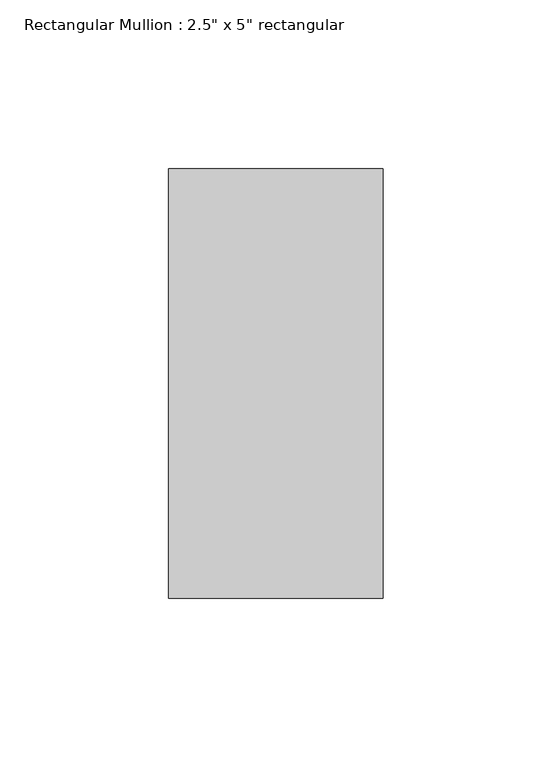
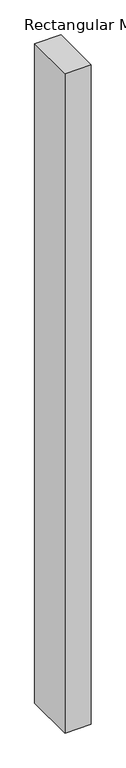
"""IFC4 building model written with IfcOpenShell, lengths in millimetres: member geometry."""

from ifc_helpers import new_model, si_unit, frame, origin, place, context, project, spatial, polyline, outline, extrude, source, transform, mapped, element, save


def member_fe0bf6b7(model_context):
    return source(origin(), model_context, "Body", "SweptSolid", [
        extrude(outline(polyline([(0.0, 63.5), (0.0, -63.5), (-63.5, -63.5), (-63.5, 63.5), (0.0, 63.5)])), frame((0.0, 0.0, -1696.2528693), z_axis=(0.0, 0.0, 1.0), x_axis=(1.0, 0.0, 0.0)), (0.0, 0.0, 1.0), 1696.2528693),
    ])


if __name__ == "__main__":
    model = new_model("IFC4")
    model_context = context("Model", 3, world=origin())
    ifc_project = project(units=[si_unit("LENGTHUNIT", "METRE", prefix="MILLI")], contexts=[model_context])
    site = spatial("IfcSite", under=ifc_project)
    building = spatial("IfcBuilding", under=site)
    placement = place(None, origin())
    member_shape = member_fe0bf6b7(model_context)
    element("IfcMember", 1, ObjectType="Rectangular Mullion : 2.5\" x 5\" rectangular", at=placement, inside=building, context=model_context, shape_type="MappedRepresentation", body=[
        mapped(member_shape, transform((0.0, 0.0, 0.0), x_axis=(1.0, 0.0, 0.0), y_axis=(0.0, 1.0, 0.0), z_axis=(0.0, 0.0, 1.0))),
    ])
    save(model, "model.ifc")

# Revit data of these elements
# Type "Rectangular Mullion : 2.5\" x 5\" rectangular"
#   built-in parameter 1007304 = 0.416667 (stored number, unit not read)
#   built-in parameter 1007301 = 0.104167 (stored number, unit not read)
#   built-in parameter 1007300 = 0.104167 (stored number, unit not read)
# Element 1 (IfcMember, "Rectangular Mullion : 2.5\" x 5\" rectangular")
#   Materials on its faces: "Aluminum"
# Materials
#   "Aluminum": class "Metal", colour RGB 247 247 247, transparency 0, Description = "Aluminum 6061", Cost = 0
